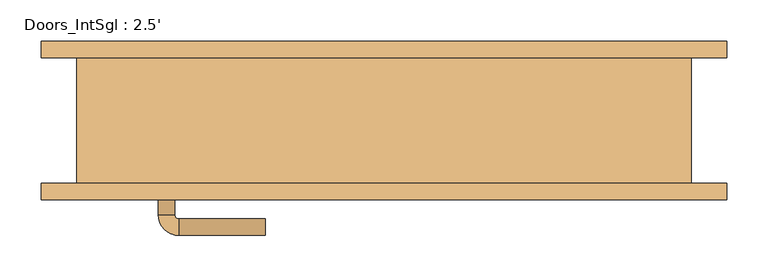
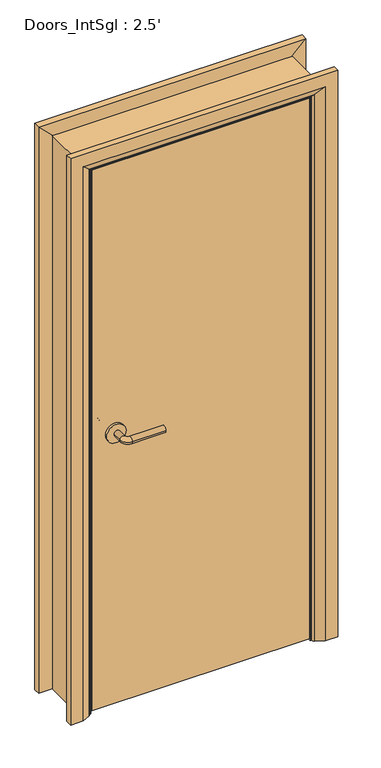
"""IFC4 building model written with IfcOpenShell, lengths in millimetres: door geometry, Doors_IntSgl : 2.5'."""

from ifc_helpers import new_model, si_unit, point, frame, frame_2d, origin, place, context, project, spatial, polyline, circle_curve, ellipse_curve, trimmed, segment, composite_curve, outline, extrude, faceted_brep, source, transform, mapped, element, save
from ifc_brep_helpers import plane_surface, cylinder_surface, revolved_surface, advanced_brep


def doors_intsgl_2_5_55235da4(model_context):
    return source(origin(), model_context, "Body", "SolidModel", [
        advanced_brep(
        [(-274.0, -30.2, 900.0), (-254.0, -30.2, 900.0), (-274.0, -0.2, 900.0), (-254.0, -0.2, 900.0), (-249.0, 4.8, 900.0), (-249.0, 24.8, 900.0), (-144.0, 24.8, 900.0), (-144.0, 4.8, 900.0)],
        [
            (0, 1, circle_curve(frame((-264.0, -30.2, 900.0), z_axis=(0.0, -1.0, 0.0), x_axis=(1.0, 0.0, 0.0)), 10.0)),
            (1, 0, circle_curve(frame((-264.0, -30.2, 900.0), z_axis=(0.0, -1.0, 0.0), x_axis=(1.0, 0.0, 0.0)), 10.0)),
            (0, 2),
            (2, 3, circle_curve(frame((-264.0, -0.2, 900.0), z_axis=(0.0, -1.0, 0.0), x_axis=(1.0, 0.0, 0.0)), 10.0)),
            (3, 1),
            (3, 2, circle_curve(frame((-264.0, -0.2, 900.0), z_axis=(0.0, -1.0, 0.0), x_axis=(1.0, 0.0, 0.0)), 10.0)),
            (4, 3, circle_curve(frame((-249.0, -0.2, 900.0), z_axis=(0.0, 0.0, 1.0), x_axis=(-1.0, 0.0, 0.0)), 5.0)),
            (2, 5, circle_curve(frame((-249.0, -0.2, 900.0), z_axis=(0.0, 0.0, -1.0), x_axis=(-1.0, 0.0, 0.0)), 25.0)),
            (5, 4, circle_curve(frame((-249.0, 14.8, 900.0), z_axis=(-1.0, 0.0, 0.0), x_axis=(0.0, -1.0, 0.0)), 10.0)),
            (4, 5, circle_curve(frame((-249.0, 14.8, 900.0), z_axis=(-1.0, 0.0, 0.0), x_axis=(0.0, -1.0, 0.0)), 10.0)),
            (6, 7, circle_curve(frame((-144.0, 14.8, 900.0), z_axis=(1.0, 0.0, 0.0), x_axis=(0.0, -1.0, 0.0)), 10.0)),
            (7, 6, circle_curve(frame((-144.0, 14.8, 900.0), z_axis=(1.0, 0.0, 0.0), x_axis=(0.0, -1.0, 0.0)), 10.0)),
            (5, 6),
            (7, 4),
        ],
        [
            plane_surface(frame((-264.0, -30.2, 900.0), z_axis=(0.0, -1.0, 0.0), x_axis=(0.0, 0.0, 1.0))),
            cylinder_surface(frame((-264.0, -30.2, 900.0), z_axis=(0.0, -1.0, 0.0), x_axis=(1.0, 0.0, 0.0)), 10.0),
            revolved_surface(trimmed(ellipse_curve(frame((-264.0, -0.2, 900.0), z_axis=(0.0, -1.0, 0.0), x_axis=(1.0, 0.0, 0.0)), 10.0, 10.0), [point((-274.0, -0.2, 900.0))], [point((-254.0, -0.2, 900.0))], True, "CARTESIAN"), (-249.0, -0.2, 900.0), (0.0, 0.0, -1.0)),
            revolved_surface(trimmed(ellipse_curve(frame((-264.0, -0.2, 900.0), z_axis=(0.0, -1.0, 0.0), x_axis=(1.0, 0.0, 0.0)), 10.0, 10.0), [point((-254.0, -0.2, 900.0))], [point((-274.0, -0.2, 900.0))], True, "CARTESIAN"), (-249.0, -0.2, 900.0), (0.0, 0.0, -1.0)),
            plane_surface(frame((-144.0, 14.8, 900.0), z_axis=(1.0, 0.0, 0.0), x_axis=(0.0, 0.0, 1.0))),
            cylinder_surface(frame((-249.0, 14.8, 900.0), z_axis=(-1.0, 0.0, 0.0), x_axis=(0.0, -1.0, 0.0)), 10.0),
        ],
        [
            (0, [[1, 2]]),
            (1, [[-1, 3, 4, 5]]),
            (1, [[-2, -5, 6, -3]]),
            (2, [[7, -4, 8, 9]]),
            (3, [[-8, -6, -7, 10]]),
            (4, [[11, 12]]),
            (5, [[-9, 13, -12, 14]]),
            (5, [[-10, -14, -11, -13]]),
        ],
    ),
        extrude(outline(composite_curve([segment(trimmed(circle_curve(frame_2d((900.0, -266.5)), 30.0), [point((900.0, -296.5))], [point((900.0, -236.5))], False, "CARTESIAN"), True, "CONTINUOUS"), segment(trimmed(circle_curve(frame_2d((900.0, -266.5)), 30.0), [point((900.0, -236.5))], [point((900.0, -296.5))], False, "CARTESIAN"), True, "CONTINUOUS")], self_intersect=False)), frame((0.0, -38.2, 0.0), z_axis=(0.0, 1.0, 0.0), x_axis=(0.0, 0.0, 1.0)), (0.0, 0.0, 1.0), 8.0),
        advanced_brep(
        [(-274.0, -84.2, 900.0), (-254.0, -84.2, 900.0), (-254.0, -114.2, 900.0), (-274.0, -114.2, 900.0), (-249.0, -119.2, 900.0), (-249.0, -139.2, 900.0), (-144.0, -139.2, 900.0), (-144.0, -119.2, 900.0)],
        [
            (0, 1, circle_curve(frame((-264.0, -84.2, 900.0), z_axis=(0.0, 1.0, 0.0), x_axis=(1.0, 0.0, 0.0)), 10.0)),
            (1, 0, circle_curve(frame((-264.0, -84.2, 900.0), z_axis=(0.0, 1.0, 0.0), x_axis=(1.0, 0.0, 0.0)), 10.0)),
            (1, 2),
            (2, 3, circle_curve(frame((-264.0, -114.2, 900.0), z_axis=(0.0, 1.0, 0.0), x_axis=(1.0, 0.0, 0.0)), 10.0)),
            (3, 0),
            (3, 2, circle_curve(frame((-264.0, -114.2, 900.0), z_axis=(0.0, 1.0, 0.0), x_axis=(1.0, 0.0, 0.0)), 10.0)),
            (4, 5, circle_curve(frame((-249.0, -129.2, 900.0), z_axis=(-1.0, 0.0, 0.0), x_axis=(0.0, 1.0, 0.0)), 10.0)),
            (5, 3, circle_curve(frame((-249.0, -114.2, 900.0), z_axis=(0.0, 0.0, -1.0), x_axis=(-1.0, 0.0, 0.0)), 25.0)),
            (2, 4, circle_curve(frame((-249.0, -114.2, 900.0), z_axis=(0.0, 0.0, 1.0), x_axis=(-1.0, 0.0, 0.0)), 5.0)),
            (5, 4, circle_curve(frame((-249.0, -129.2, 900.0), z_axis=(-1.0, 0.0, 0.0), x_axis=(0.0, 1.0, 0.0)), 10.0)),
            (6, 7, circle_curve(frame((-144.0, -129.2, 900.0), z_axis=(1.0, 0.0, 0.0), x_axis=(0.0, 1.0, 0.0)), 10.0)),
            (7, 6, circle_curve(frame((-144.0, -129.2, 900.0), z_axis=(1.0, 0.0, 0.0), x_axis=(0.0, 1.0, 0.0)), 10.0)),
            (4, 7),
            (6, 5),
        ],
        [
            plane_surface(frame((-264.0, -84.2, 900.0), z_axis=(0.0, 1.0, 0.0), x_axis=(0.0, 0.0, 1.0))),
            cylinder_surface(frame((-264.0, -84.2, 900.0), z_axis=(0.0, 1.0, 0.0), x_axis=(1.0, 0.0, 0.0)), 10.0),
            revolved_surface(trimmed(ellipse_curve(frame((-264.0, -114.2, 900.0), z_axis=(0.0, -1.0, 0.0), x_axis=(1.0, 0.0, 0.0)), 10.0, 10.0), [point((-274.0, -114.2, 900.0))], [point((-254.0, -114.2, 900.0))], True, "CARTESIAN"), (-249.0, -114.2, 900.0), (0.0, 0.0, -1.0)),
            revolved_surface(trimmed(ellipse_curve(frame((-264.0, -114.2, 900.0), z_axis=(0.0, -1.0, 0.0), x_axis=(1.0, 0.0, 0.0)), 10.0, 10.0), [point((-254.0, -114.2, 900.0))], [point((-274.0, -114.2, 900.0))], True, "CARTESIAN"), (-249.0, -114.2, 900.0), (0.0, 0.0, -1.0)),
            plane_surface(frame((-144.0, -129.2, 900.0), z_axis=(1.0, 0.0, 0.0), x_axis=(0.0, 0.0, 1.0))),
            cylinder_surface(frame((-249.0, -129.2, 900.0), z_axis=(-1.0, 0.0, 0.0), x_axis=(0.0, 1.0, 0.0)), 10.0),
        ],
        [
            (0, [[1, 2]]),
            (1, [[3, 4, 5, -2]]),
            (1, [[-5, 6, -3, -1]]),
            (2, [[7, 8, -4, 9]]),
            (3, [[10, -9, -6, -8]]),
            (4, [[11, 12]]),
            (5, [[13, -11, 14, -7]]),
            (5, [[-14, -12, -13, -10]]),
        ],
    ),
        extrude(outline(composite_curve([segment(trimmed(circle_curve(frame_2d((900.0, -266.5)), 30.0), [point((900.0, -296.5))], [point((900.0, -236.5))], False, "CARTESIAN"), True, "CONTINUOUS"), segment(trimmed(circle_curve(frame_2d((900.0, -266.5)), 30.0), [point((900.0, -236.5))], [point((900.0, -296.5))], False, "CARTESIAN"), True, "CONTINUOUS")], self_intersect=False)), frame((0.0, -84.2, 0.0), z_axis=(0.0, 1.0, 0.0), x_axis=(0.0, 0.0, 1.0)), (0.0, 0.0, 1.0), 8.0),
        extrude(outline(polyline([(339.0, -38.2), (339.0, -76.2), (-339.0, -76.2), (-339.0, -38.2), (339.0, -38.2)])), frame((0.0, 0.0, 8.0), z_axis=(0.0, 0.0, 1.0), x_axis=(1.0, 0.0, 0.0)), (0.0, 0.0, 1.0), 1778.8),
        advanced_brep(
        [(416.0, -96.2, 0.0), (376.0, -96.2, 0.0), (350.0, -82.2, 0.0), (346.0, -76.2, 0.0), (416.0, -76.2, 0.0), (416.0, -76.2, 1863.8), (416.0, -96.2, 1863.8), (346.0, -76.2, 1793.8), (-346.0, -76.2, 1793.8), (-346.0, -76.2, 0.0), (-416.0, -76.2, 0.0), (-416.0, -76.2, 1863.8), (350.0, -82.2, 1797.8), (376.0, -96.2, 1823.8), (-416.0, -96.2, 1863.8), (-416.0, -96.2, 0.0), (-376.0, -96.2, 0.0), (-376.0, -96.2, 1823.8), (-350.0, -82.2, 0.0), (-350.0, -82.2, 1797.8)],
        [
            (0, 1),
            (1, 2),
            (2, 3, circle_curve(frame((354.0, -75.2, 0.0), z_axis=(0.0, 0.0, -1.0), x_axis=(1.0, 0.0, 0.0)), 8.0622577)),
            (3, 4),
            (4, 0),
            (4, 5),
            (5, 6),
            (6, 0),
            (3, 7),
            (7, 8),
            (8, 9),
            (9, 10),
            (10, 11),
            (11, 5),
            (2, 12),
            (12, 7, ellipse_curve(frame((354.0, -75.2, 1801.8), z_axis=(0.7071067811865475, 0.0, -0.7071067811865475), x_axis=(-0.7071067811865474, 0.0, -0.7071067811865476)), 11.4017543, 8.0622577)),
            (1, 13),
            (13, 12),
            (6, 14),
            (14, 15),
            (15, 16),
            (16, 17),
            (17, 13),
            (10, 15),
            (14, 11),
            (9, 18, circle_curve(frame((-354.0, -75.2, 0.0), z_axis=(0.0, 0.0, -1.0), x_axis=(-1.0, 0.0, 0.0)), 8.0622577)),
            (18, 16),
            (19, 18),
            (8, 19, ellipse_curve(frame((-354.0, -75.2, 1801.8), z_axis=(-0.7071067811865475, 0.0, -0.7071067811865475), x_axis=(-0.7071067811865474, 0.0, 0.7071067811865476)), 11.4017543, 8.0622577)),
            (19, 17),
            (12, 19),
        ],
        [
            plane_surface(frame((346.0, -76.2, 0.0), z_axis=(0.0, 0.0, -1.0), x_axis=(0.0, 1.0, 0.0))),
            plane_surface(frame((416.0, -96.2, 0.0), z_axis=(1.0, 0.0, 0.0), x_axis=(0.0, 0.0, 1.0))),
            plane_surface(frame((416.0, -76.2, 0.0), z_axis=(0.0, 1.0, 0.0), x_axis=(0.0, 0.0, 1.0))),
            cylinder_surface(frame((354.0, -75.2, 0.0), z_axis=(0.0, 0.0, -1.0), x_axis=(1.0, 0.0, 0.0)), 8.0622577),
            plane_surface(frame((350.0, -82.2, 0.0), z_axis=(-0.4740998230350126, -0.880471099922178, 0.0), x_axis=(0.0, 0.0, 1.0))),
            plane_surface(frame((376.0, -96.2, 0.0), z_axis=(0.0, -1.0, 0.0), x_axis=(0.0, 0.0, 1.0))),
            plane_surface(frame((-416.0, -96.2, 1863.8), z_axis=(-1.0, 0.0, 0.0), x_axis=(0.0, 0.0, -1.0))),
            plane_surface(frame((-346.0, -76.2, 0.0), z_axis=(0.0, 0.0, -1.0), x_axis=(0.0, 1.0, 0.0))),
            cylinder_surface(frame((-354.0, -75.2, 1793.8), z_axis=(0.0, 0.0, 1.0), x_axis=(-1.0, 0.0, 0.0)), 8.0622577),
            plane_surface(frame((-350.0, -82.2, 1797.8), z_axis=(0.47409982303501824, -0.8804710999221749, 0.0), x_axis=(0.0, 0.0, -1.0))),
            plane_surface(frame((416.0, -96.2, 1863.8), z_axis=(0.0, 0.0, 1.0), x_axis=(-1.0, 0.0, 0.0))),
            cylinder_surface(frame((346.0, -75.2, 1801.8), z_axis=(1.0, 0.0, 0.0), x_axis=(0.0, 0.0, 1.0)), 8.0622577),
            plane_surface(frame((350.0, -82.2, 1797.8), z_axis=(0.0, -0.8804710999221764, -0.4740998230350154), x_axis=(-1.0, 0.0, 0.0))),
        ],
        [
            (0, [[1, 2, 3, 4, 5]]),
            (1, [[6, 7, 8, -5]]),
            (2, [[9, 10, 11, 12, 13, 14, -6, -4]]),
            (3, [[15, 16, -9, -3]]),
            (4, [[17, 18, -15, -2]]),
            (5, [[-8, 19, 20, 21, 22, 23, -17, -1]]),
            (6, [[-13, 24, -20, 25]]),
            (7, [[-24, -12, 26, 27, -21]]),
            (8, [[28, -26, -11, 29]]),
            (9, [[-22, -27, -28, 30]]),
            (10, [[-14, -25, -19, -7]]),
            (11, [[31, -29, -10, -16]]),
            (12, [[-23, -30, -31, -18]]),
        ],
    ),
        extrude(outline(polyline([(0.0, -322.0), (1769.8, -322.0), (1769.8, 322.0), (0.0, 322.0), (0.0, 341.0), (1788.8, 341.0), (1788.8, -341.0), (0.0, -341.0), (0.0, -322.0)])), frame((0.0, -36.2, 0.0), z_axis=(0.0, 1.0, 0.0), x_axis=(0.0, 0.0, 1.0)), (0.0, 0.0, 1.0), 32.0),
        advanced_brep(
        [(-416.0, 96.2, 0.0), (-376.0, 96.2, 0.0), (-350.0, 82.2, 0.0), (-346.0, 76.2, 0.0), (-416.0, 76.2, 0.0), (-416.0, 76.2, 1863.8), (-416.0, 96.2, 1863.8), (-346.0, 76.2, 1793.8), (-350.0, 82.2, 1797.8), (-376.0, 96.2, 1823.8), (416.0, 96.2, 0.0), (416.0, 76.2, 0.0), (346.0, 76.2, 0.0), (350.0, 82.2, 0.0), (376.0, 96.2, 0.0), (416.0, 96.2, 1863.8), (376.0, 96.2, 1823.8), (350.0, 82.2, 1797.8), (346.0, 76.2, 1793.8), (416.0, 76.2, 1863.8)],
        [
            (0, 1),
            (1, 2),
            (2, 3, circle_curve(frame((-354.0, 75.2, 0.0), z_axis=(0.0, 0.0, -1.0), x_axis=(-1.0, 0.0, 0.0)), 8.0622577)),
            (3, 4),
            (4, 0),
            (4, 5),
            (5, 6),
            (6, 0),
            (3, 7),
            (7, 5),
            (2, 8),
            (8, 7, ellipse_curve(frame((-354.0, 75.2, 1801.8), z_axis=(-0.7071067811865475, 0.0, -0.7071067811865475), x_axis=(0.7071067811865474, 0.0, -0.7071067811865476)), 11.4017543, 8.0622577)),
            (1, 9),
            (9, 8),
            (6, 9),
            (10, 11),
            (11, 12),
            (12, 13, circle_curve(frame((354.0, 75.2, 0.0), z_axis=(0.0, 0.0, -1.0), x_axis=(1.0, 0.0, 0.0)), 8.0622577)),
            (13, 14),
            (14, 10),
            (15, 10),
            (14, 16),
            (16, 15),
            (13, 17),
            (17, 16),
            (12, 18),
            (18, 17, ellipse_curve(frame((354.0, 75.2, 1801.8), z_axis=(0.7071067811865475, 0.0, -0.7071067811865475), x_axis=(0.7071067811865474, 0.0, 0.7071067811865476)), 11.4017543, 8.0622577)),
            (11, 19),
            (19, 18),
            (15, 19),
            (5, 19),
            (15, 6),
            (7, 18),
            (8, 17),
            (9, 16),
        ],
        [
            plane_surface(frame((-346.0, 149.0010989, 0.0), z_axis=(0.0, 0.0, -1.0), x_axis=(1.0, 0.0, 0.0))),
            plane_surface(frame((-416.0, 96.2, 0.0), z_axis=(-1.0, 0.0, 0.0), x_axis=(0.0, 0.0, 1.0))),
            plane_surface(frame((-416.0, 76.2, 0.0), z_axis=(0.0, -1.0, 0.0), x_axis=(0.0, 0.0, 1.0))),
            cylinder_surface(frame((-354.0, 75.2, 0.0), z_axis=(0.0, 0.0, -1.0), x_axis=(-1.0, 0.0, 0.0)), 8.0622577),
            plane_surface(frame((-350.0, 82.2, 0.0), z_axis=(0.4740998230350183, 0.8804710999221749, 0.0), x_axis=(0.0, 0.0, 1.0))),
            plane_surface(frame((-376.0, 96.2, 0.0), z_axis=(0.0, 1.0, 0.0), x_axis=(0.0, 0.0, 1.0))),
            plane_surface(frame((346.0, 149.0010989, 0.0), z_axis=(0.0, 0.0, -1.0), x_axis=(-1.0, 0.0, 0.0))),
            plane_surface(frame((376.0, 96.2, 1823.8), z_axis=(0.0, 1.0, 0.0), x_axis=(0.0, 0.0, -1.0))),
            plane_surface(frame((350.0, 82.2, 1797.8), z_axis=(-0.4740998230350183, 0.8804710999221749, 0.0), x_axis=(0.0, 0.0, -1.0))),
            cylinder_surface(frame((354.0, 75.2, 1793.8), z_axis=(0.0, 0.0, 1.0), x_axis=(1.0, 0.0, 0.0)), 8.0622577),
            plane_surface(frame((416.0, 76.2, 1863.8), z_axis=(0.0, -1.0, 0.0), x_axis=(0.0, 0.0, -1.0))),
            plane_surface(frame((416.0, 96.2, 1863.8), z_axis=(1.0, 0.0, 0.0), x_axis=(0.0, 0.0, -1.0))),
            plane_surface(frame((-416.0, 96.2, 1863.8), z_axis=(0.0, 0.0, 1.0), x_axis=(1.0, 0.0, 0.0))),
            plane_surface(frame((-416.0, 76.2, 1863.8), z_axis=(0.0, -1.0, 0.0), x_axis=(1.0, 0.0, 0.0))),
            cylinder_surface(frame((-346.0, 75.2, 1801.8), z_axis=(-1.0, 0.0, 0.0), x_axis=(0.0, 0.0, 1.0)), 8.0622577),
            plane_surface(frame((-350.0, 82.2, 1797.8), z_axis=(0.0, 0.8804710999221749, -0.4740998230350183), x_axis=(1.0, 0.0, 0.0))),
            plane_surface(frame((-376.0, 96.2, 1823.8), z_axis=(0.0, 1.0, 0.0), x_axis=(1.0, 0.0, 0.0))),
        ],
        [
            (0, [[1, 2, 3, 4, 5]]),
            (1, [[6, 7, 8, -5]]),
            (2, [[9, 10, -6, -4]]),
            (3, [[11, 12, -9, -3]]),
            (4, [[13, 14, -11, -2]]),
            (5, [[-8, 15, -13, -1]]),
            (6, [[16, 17, 18, 19, 20]]),
            (7, [[21, -20, 22, 23]]),
            (8, [[-22, -19, 24, 25]]),
            (9, [[-24, -18, 26, 27]]),
            (10, [[-26, -17, 28, 29]]),
            (11, [[-28, -16, -21, 30]]),
            (12, [[31, -30, 32, -7]]),
            (13, [[33, -29, -31, -10]]),
            (14, [[34, -27, -33, -12]]),
            (15, [[35, -25, -34, -14]]),
            (16, [[-32, -23, -35, -15]]),
        ],
    ),
        faceted_brep([(-341.0, -76.2, 0.0), (-373.0, -76.2, 0.0), (-373.0, 76.2, 0.0), (-341.0, 76.2, 0.0), (-341.0, 76.2, 1788.8), (-341.0, -76.2, 1788.8), (-373.0, 76.2, 1820.8), (-373.0, -76.2, 1820.8), (341.0, -76.2, 0.0), (341.0, 76.2, 0.0), (373.0, 76.2, 0.0), (373.0, -76.2, 0.0), (341.0, -76.2, 1788.8), (373.0, -76.2, 1820.8), (373.0, 76.2, 1820.8), (341.0, 76.2, 1788.8)], [[[0, 1, 2, 3]], [[3, 4, 5, 0]], [[2, 6, 4, 3]], [[1, 7, 6, 2]], [[0, 5, 7, 1]], [[8, 9, 10, 11]], [[12, 8, 11, 13]], [[13, 11, 10, 14]], [[14, 10, 9, 15]], [[15, 9, 8, 12]], [[4, 15, 12, 5]], [[6, 14, 15, 4]], [[7, 13, 14, 6]], [[5, 12, 13, 7]]]),
    ])


if __name__ == "__main__":
    model = new_model("IFC4")
    model_context = context("Model", 3, world=origin())
    ifc_project = project(units=[si_unit("LENGTHUNIT", "METRE", prefix="MILLI")], contexts=[model_context])
    site = spatial("IfcSite", under=ifc_project)
    building = spatial("IfcBuilding", under=site)
    placement = place(None, origin())
    doors_intsgl_2_5_shape = doors_intsgl_2_5_55235da4(model_context)
    element("IfcDoor", 1, ObjectType="Doors_IntSgl : 2.5'", at=placement, inside=building, context=model_context, shape_type="MappedRepresentation", body=[
        mapped(doors_intsgl_2_5_shape, transform((0.0, 0.0, 0.0), x_axis=(1.0, 0.0, 0.0), y_axis=(0.0, 1.0, 0.0), z_axis=(0.0, 0.0, 1.0))),
    ])
    save(model, "model.ifc")

# Revit data of these elements
# Type "Doors_IntSgl : 2.5'"
#   Type Mark = "49"
#   Type Comments = "Internal Single"
#   Operation = "SingleSwingRight"
#   Manufacturer = "Revit"
#   Keynote = "L20"
#   Description = "Internal Single Door"
#   Analytic Construction = "Metal"
#   UnderCut = 0' - 0.31496"
#   Tolerance = 0' - 0.07874"
#   Thickness = 0' - 1.49606"
#   Thermal Resistance (R) = 0.270117 (m²·K)/W
#   Structural Tolerance = 0' - 0.31496"
#   StopDepth = 0' - 1.25984"
#   Stop Thickness = 0' - 0.74803"
#   Rough Width = 2' - 6"
#   Rough Height = 6' - 0"
#   Height to Top Lock Rail = 3' - 3.37008"
#   Heat Transfer Coefficient (U) = 3.7021 W/(m²·K)
#   Handle Z Distance = 2' - 11.43307"
#   Handle X Distance = 0' - 2.95276"
#   Frame Thickness = 0' - 1.25984"
#   Door Panel Width = 2' - 2.69291"
#   Door Panel Thickness = 0' - 1.49606"
#   Door Panel Offset = 0' - 0"
#   Height = 6' - 0"
#   Width = 2' - 6"
#   Door Panel Height = 5' - 10.0315"
#   Architrave Setback = 0' - 0.19685"
#   Vis - Ironmongery = yes
#   Material Ironmongery = Door - Handle
#   Material Frame = Door - Frame/Mullion (1)
#   Material Door = Door - Panel
#   Material Architrave = Door - Architrave
#   Visual Light Transmittance = 0
#   Solar Heat Gain Coefficient = 0
#   Function = (empty or 0)
#   Wall Closure = (empty or 0)
# Element 1 (IfcDoor, "Doors_IntSgl : 2.5'")
#   Materials on its faces: "Door - Architrave", "Door - Handle", "Door - Frame/Mullion (1)", "Door - Panel"
# Materials
#   "Door - Handle": colour RGB 0 0 0, transparency 0, Keynote = "P21", Cost = 0
#   "Door - Frame/Mullion (1)": class "Wood", colour RGB 212 179 113, transparency 0, Keynote = "L20", Cost = 0
#   "Door - Panel": class "Wood", colour RGB 210 159 95, transparency 0, Keynote = "L20", Cost = 0
#   "Door - Architrave": class "Wood", colour RGB 154 90 5, transparency 0, Keynote = "P20", Cost = 0
